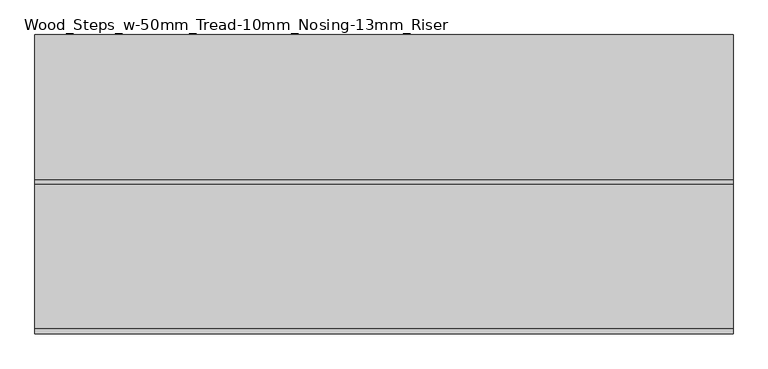
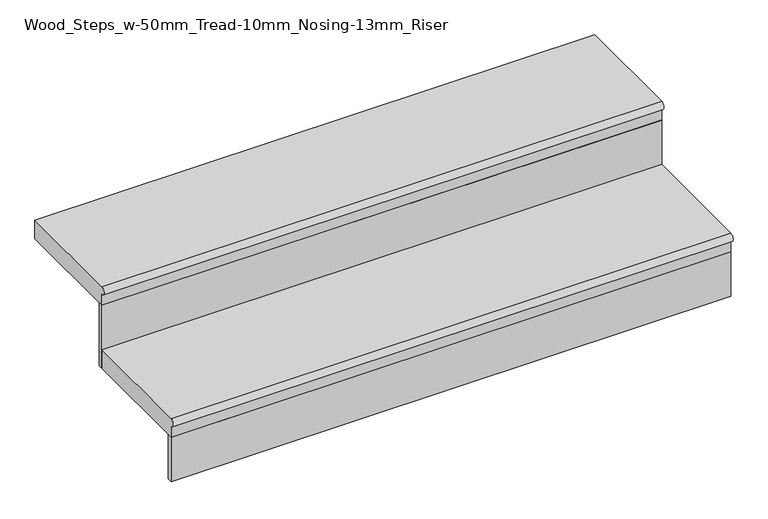
"""IFC4 building model written with IfcOpenShell, lengths in millimetres: stair flight geometry, Wood_Steps_w-50mm_Tread-10mm_Nosing-13mm_Riser."""

from ifc_helpers import new_model, si_unit, point, frame, frame_2d, origin, origin_with_axes, place, context, project, spatial, polyline, circle_curve, trimmed, segment, composite_curve, outline, extrude, source, transform, mapped, element, save


def wood_steps_w_50mm_tread_10mm_nosing_13mm_riser_33fa0412(model_context):
    return source(origin(), model_context, "Body", "SweptSolid", [
        extrude(outline(composite_curve([segment(polyline([(1076.0472041, 169.3333333), (1380.8472041, 169.3333333), (1380.8472041, 119.3333333), (1076.0472041, 119.3333333), (1076.0472041, 149.3333333)]), True, "CONTINUOUS"), segment(trimmed(circle_curve(frame_2d((1076.0472041, 159.3333333)), 10.0), [point((1076.0472041, 149.3333333))], [point((1076.0472041, 169.3333333))], False, "CARTESIAN"), True, "CONTINUOUS")], self_intersect=False)), frame((4385.1747157, 0.0, 0.0), z_axis=(1.0, 0.0, 0.0), x_axis=(0.0, 1.0, 0.0)), (0.0, 0.0, 1.0), 1422.4),
        extrude(outline(polyline([(5807.5747157, 1088.5472041), (5807.5747157, 1076.0472041), (4385.1747157, 1076.0472041), (4385.1747157, 1088.5472041), (5807.5747157, 1088.5472041)])), origin_with_axes(), (0.0, 0.0, 1.0), 119.3333333),
        extrude(outline(polyline([(5807.5747157, 1393.3472041), (5807.5747157, 1380.8472041), (4385.1747157, 1380.8472041), (4385.1747157, 1393.3472041), (5807.5747157, 1393.3472041)])), frame((0.0, 0.0, 119.3333333), z_axis=(0.0, 0.0, 1.0), x_axis=(1.0, 0.0, 0.0)), (0.0, 0.0, 1.0), 169.3333333),
        extrude(outline(composite_curve([segment(polyline([(1380.8472041, 338.6666667), (1675.6472041, 338.6666667), (1675.6472041, 288.6666667), (1380.8472041, 288.6666667), (1380.8472041, 318.6666667)]), True, "CONTINUOUS"), segment(trimmed(circle_curve(frame_2d((1380.8472041, 328.6666667)), 10.0), [point((1380.8472041, 318.6666667))], [point((1380.8472041, 338.6666667))], False, "CARTESIAN"), True, "CONTINUOUS")], self_intersect=False)), frame((4385.1747157, 0.0, 0.0), z_axis=(1.0, 0.0, 0.0), x_axis=(0.0, 1.0, 0.0)), (0.0, 0.0, 1.0), 1422.4),
    ])


if __name__ == "__main__":
    model = new_model("IFC4")
    model_context = context("Model", 3, world=origin())
    ifc_project = project(units=[si_unit("LENGTHUNIT", "METRE", prefix="MILLI")], contexts=[model_context])
    site = spatial("IfcSite", under=ifc_project)
    building = spatial("IfcBuilding", under=site)
    placement = place(None, origin())
    wood_steps_w_50mm_tread_10mm_nosing_13mm_riser_shape = wood_steps_w_50mm_tread_10mm_nosing_13mm_riser_33fa0412(model_context)
    element("IfcStairFlight", 1, ObjectType="Wood_Steps_w-50mm_Tread-10mm_Nosing-13mm_Riser", at=placement, inside=building, context=model_context, shape_type="MappedRepresentation", body=[
        mapped(wood_steps_w_50mm_tread_10mm_nosing_13mm_riser_shape, transform((0.0, 0.0, 0.0), x_axis=(1.0, 0.0, 0.0), y_axis=(0.0, 1.0, 0.0), z_axis=(0.0, 0.0, 1.0))),
    ])
    save(model, "model.ifc")

# Revit data of these elements
# Element 1 (IfcStairFlight, "Wood_Steps_w-50mm_Tread-10mm_Nosing-13mm_Riser")
#   Materials on its faces: "Oak Flooring"
# Materials
#   "Oak Flooring": class "Wood", colour RGB 212 179 113, transparency 0, Description = "Quercus Rubra", Cost = 0
